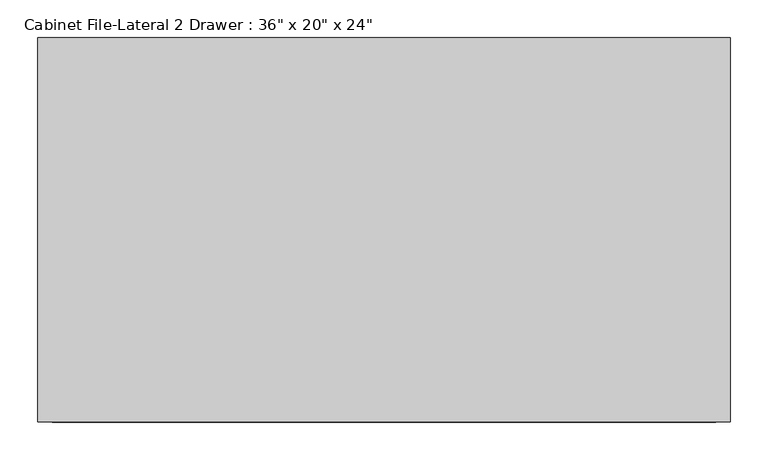
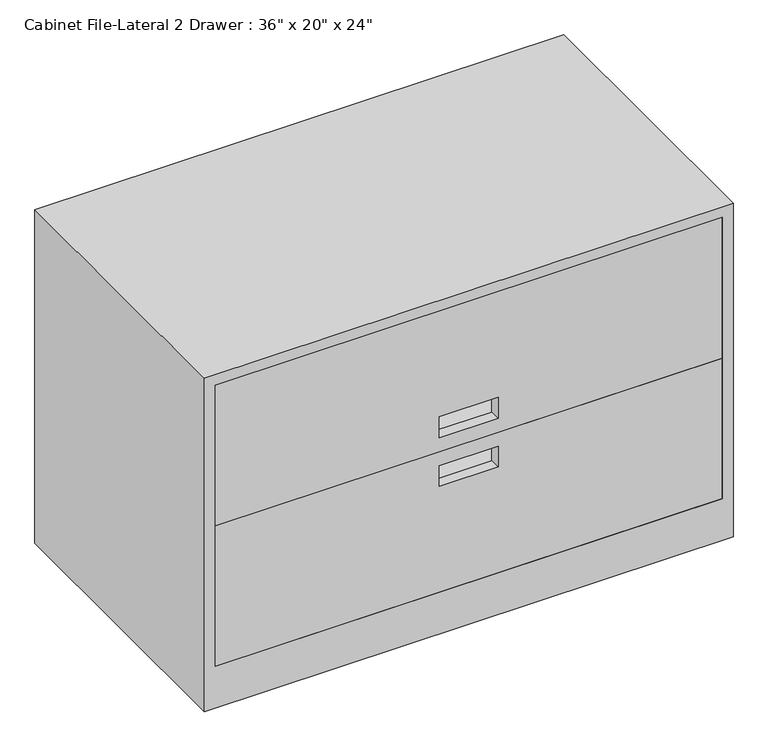
"""IFC4 building model written with IfcOpenShell, lengths in millimetres: furniture geometry."""

from ifc_helpers import new_model, si_unit, frame, origin, place, context, project, spatial, polyline, outline, extrude, faceted_brep, source, transform, mapped, element, save


def furniture_6b884072(model_context):
    return source(origin(), model_context, "Body", "SolidModel", [
        faceted_brep([(277.1774861, -680.3183761, 609.6), (-637.2225139, -680.3183761, 609.6), (-637.2225139, -1188.3183761, 609.6), (277.1774861, -1188.3183761, 609.6), (277.1774861, -680.3183761, 0.0), (277.1774861, -1188.3183761, 0.0), (-637.2225139, -1188.3183761, 0.0), (-637.2225139, -680.3183761, 0.0), (258.1274861, -1188.3183761, 76.2), (-618.1725139, -1188.3183761, 76.2), (-618.1725139, -1188.3183761, 590.55), (258.1274861, -1188.3183761, 590.55), (-618.1725139, -699.3683761, 76.2), (258.1274861, -699.3683761, 76.2), (258.1274861, -699.3683761, 590.55), (-618.1725139, -699.3683761, 590.55)], [[[0, 1, 2, 3]], [[4, 5, 6, 7]], [[1, 0, 4, 7]], [[2, 1, 7, 6]], [[3, 2, 6, 5], [8, 9, 10, 11]], [[0, 3, 5, 4]], [[12, 13, 14, 15]], [[13, 12, 9, 8]], [[14, 13, 8, 11]], [[15, 14, 11, 10]], [[12, 15, 10, 9]]]),
        extrude(outline(polyline([(333.375, -618.1725139), (333.375, 258.1274861), (590.55, 258.1274861), (590.55, -618.1725139), (333.375, -618.1725139)]), holes=[polyline([(396.875, -230.8225139), (396.875, -129.2225139), (358.775, -129.2225139), (358.775, -230.8225139), (396.875, -230.8225139)])]), frame((0.0, -1188.3183761, 0.0), z_axis=(0.0, 1.0, 0.0), x_axis=(0.0, 0.0, 1.0)), (0.0, 0.0, 1.0), 19.05),
        extrude(outline(polyline([(76.2, -618.1725139), (76.2, 258.1274861), (333.375, 258.1274861), (333.375, -618.1725139), (76.2, -618.1725139)]), holes=[polyline([(307.975, -230.8225139), (307.975, -129.2225139), (269.875, -129.2225139), (269.875, -230.8225139), (307.975, -230.8225139)])]), frame((0.0, -1188.3183761, 0.0), z_axis=(0.0, 1.0, 0.0), x_axis=(0.0, 0.0, 1.0)), (0.0, 0.0, 1.0), 19.05),
    ])


if __name__ == "__main__":
    model = new_model("IFC4")
    model_context = context("Model", 3, world=origin())
    ifc_project = project(units=[si_unit("LENGTHUNIT", "METRE", prefix="MILLI")], contexts=[model_context])
    site = spatial("IfcSite", under=ifc_project)
    building = spatial("IfcBuilding", under=site)
    placement = place(None, origin())
    furniture_shape = furniture_6b884072(model_context)
    element("IfcFurniture", 1, ObjectType="Cabinet File-Lateral 2 Drawer : 36\" x 20\" x 24\"", at=placement, inside=building, context=model_context, shape_type="MappedRepresentation", body=[
        mapped(furniture_shape, transform((0.0, 0.0, 0.0), x_axis=(1.0, 0.0, 0.0), y_axis=(0.0, 1.0, 0.0), z_axis=(0.0, 0.0, 1.0))),
    ])
    save(model, "model.ifc")

# Revit data of these elements
# Type "Cabinet File-Lateral 2 Drawer : 36\" x 20\" x 24\""
#   Assembly Code = "E2020200"
#   Depth = 1' - 8"
#   Height = 2' - 0"
#   Width = 3' - 0"
#   Material = Metal - Steel
#   Default Elevation = 0
# Element 1 (IfcFurniture, "Cabinet File-Lateral 2 Drawer : 36\" x 20\" x 24\"")
#   Materials on its faces: "Metal - Steel"
# Materials
#   "Metal - Steel": colour RGB 210 210 210, transparency 0
